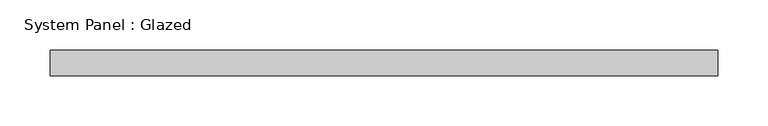
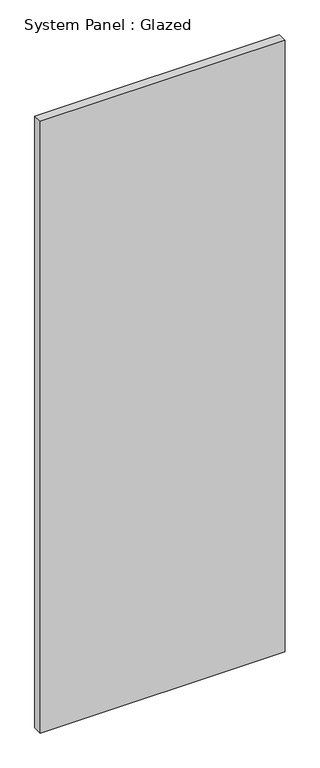
"""IFC4 building model written with IfcOpenShell, lengths in millimetres: plate geometry, System Panel : Glazed."""

from ifc_helpers import new_model, si_unit, origin, origin_with_axes, place, context, project, spatial, polyline, outline, extrude, source, transform, mapped, element, save


def system_panel_glazed_5e543223(model_context):
    return source(origin(), model_context, "Body", "SweptSolid", [
        extrude(outline(polyline([(333.375, 19.05), (-333.375, 19.05), (-333.375, 44.45), (333.375, 44.45), (333.375, 19.05)])), origin_with_axes(), (0.0, 0.0, 1.0), 1760.2910101),
    ])


if __name__ == "__main__":
    model = new_model("IFC4")
    model_context = context("Model", 3, world=origin())
    ifc_project = project(units=[si_unit("LENGTHUNIT", "METRE", prefix="MILLI")], contexts=[model_context])
    site = spatial("IfcSite", under=ifc_project)
    building = spatial("IfcBuilding", under=site)
    placement = place(None, origin())
    system_panel_glazed_shape = system_panel_glazed_5e543223(model_context)
    element("IfcPlate", 1, ObjectType="System Panel : Glazed", at=placement, inside=building, context=model_context, shape_type="MappedRepresentation", body=[
        mapped(system_panel_glazed_shape, transform((0.0, 0.0, 0.0), x_axis=(1.0, 0.0, 0.0), y_axis=(0.0, 1.0, 0.0), z_axis=(0.0, 0.0, 1.0))),
    ])
    save(model, "model.ifc")

# Revit data of these elements
# Type "System Panel : Glazed"
#   Construction Type Id = "GSP4R"
#   Analytic Construction = "1/8 in Pilkington single glazing"
#   Visual Light Transmittance = 0.9
#   Solar Heat Gain Coefficient = 0.86
#   Heat Transfer Coefficient (U) = 1.18115 BTU/(h·ft²·°F)
#   Define Thermal Properties by = 1
# Element 1 (IfcPlate, "System Panel : Glazed")
#   Materials on its faces: "Glass"
# Materials
#   "Glass": class "Glass", colour RGB 0 128 192, transparency 0.75, Description = "Soda Lime Glass", Cost = 0
